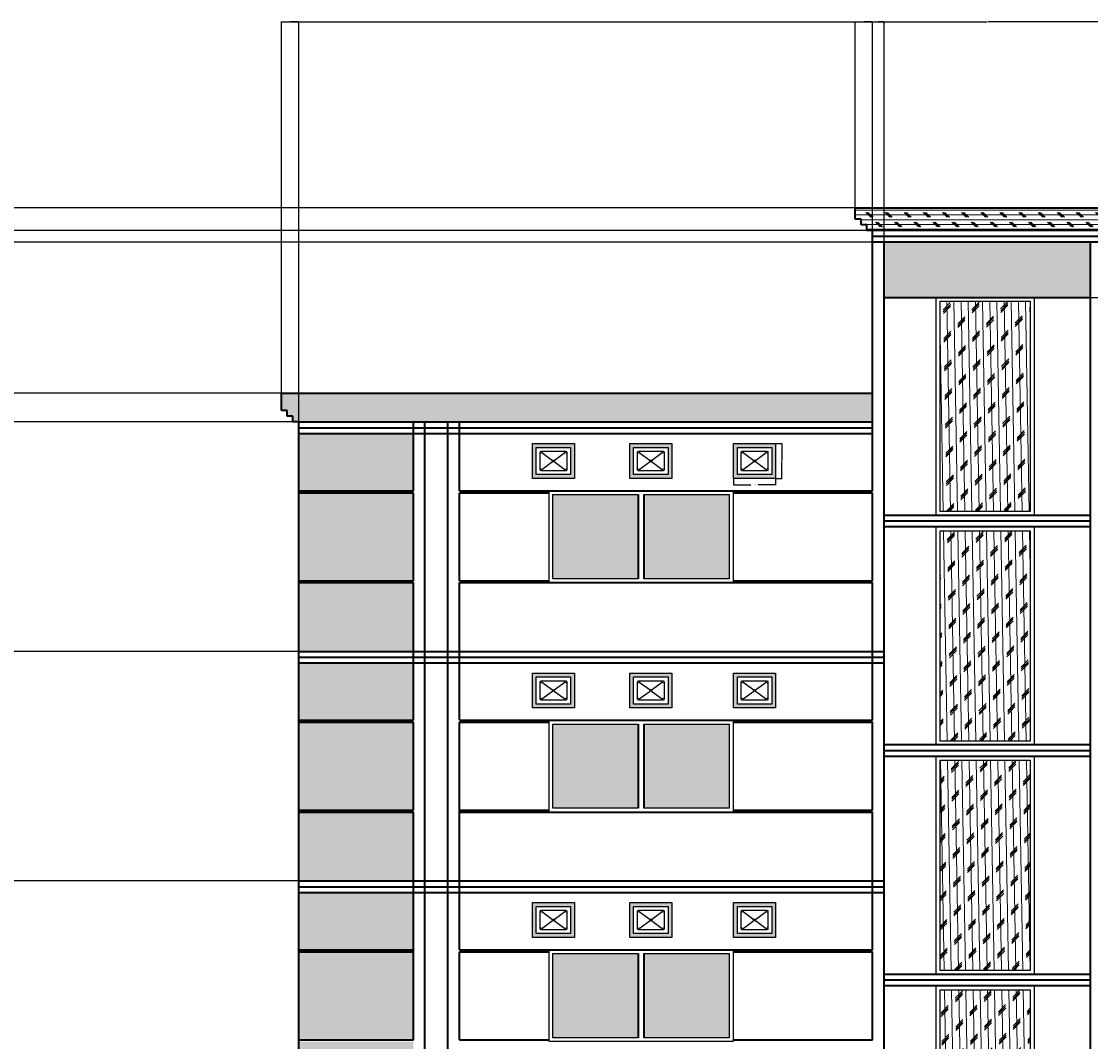
# Model space of a CAD drawing. Units: inches. Extents: x -742 to 1386, y -64 to 951.
# Tile 6 of 8: x -183 to 376, y 418 to 951. Entities that reach past the tile are written whole.
import ezdxf

# ---------------------------------------------------------------- set-up
doc = ezdxf.new("R2010")
doc.units = ezdxf.units.IN
doc.header["$MEASUREMENT"] = 0
for name, color, linetype, lineweight in [('A-ANNO-DIMS', 2, 'Continuous', 18), ('A-ELEV', 7, 'Continuous', 35), ('A-ELEV-PATT', 252, 'Continuous', 13), ('A-GLAZ', 4, 'Continuous', 25), ('A-GLAZ-PATT', 9, 'Continuous', 13), ('A-WALL-PATT', 8, 'Continuous', 13)]:
    doc.layers.add(name, color=color, linetype=linetype, lineweight=lineweight)
doc.styles.get("Standard").update_dxf_attribs({"font": 'arial.ttf'})
doc.dimstyles.get("Standard").update_dxf_attribs({"dimtxt": 0.18, "dimasz": 0.18, "dimexe": 0.18, "dimexo": 0.0625, "dimgap": 0.09, "dimtad": 0, "dimtih": 1, "dimtoh": 1, "dimdec": 4, "dimzin": 0, "dimdsep": 46, "dimtxsty": 'Standard', "dimcen": 0.09, "dimadec": 0, "dimazin": 0, "dimtfac": 1, "dimtdec": 4, "dimtofl": 0, "dimtmove": 0, "dimatfit": 3, "dimfxl": 1, "dimtolj": 1, "dimtzin": 0, "dimarcsym": 0})
pattern_1 = [(91, (0, 0), (-3.749429, -0.065447), []), (226, (1.842, 1.907), (7.62975, -7.36796), [5.3033, -5.3033]), (226, (1.826, 2.845), (7.62975, -7.36796), [5.3033, -5.3033]), (226, (1.809, 3.782), (7.62975, -7.36796), [5.3033, -5.3033])]

# ---------------------------------------------------------------- blocks, each defined once
blk = doc.blocks.new('VENT-WIN')
h = blk.add_hatch(color=256)
h.dxf.hatch_style = 1
h.paths.add_polyline_path([(11.51, 9.11, 1), (10.47, 9.11, 1)])
h.paths.add_polyline_path([(16.95, 13.71, 1), (17.99, 13.71, 1)])
h.paths.add_polyline_path([(17.99, 4.52, 1), (16.95, 4.52, 1)])
h.paths.add_polyline_path([(5.04, 4.52, 1), (4, 4.52, 1)])
h.paths.add_polyline_path([(4, 13.71, 1), (5.04, 13.71, 1)])
for p, q in [((4.99, 13.5), (10.57, 9.42)), ((11.41, 9.42), (16.99, 13.5)), ((4.99, 4.73), (10.57, 8.81)), ((11.41, 8.81), (16.99, 4.73))]:
    blk.add_line(p, q)
for points in [[(0, 18.22), (21.99, 18.22), (21.99, 0), (0, 0)], [(2, 16.22), (19.99, 16.22), (19.99, 2), (2, 2)]]:
    blk.add_lwpolyline(points, close=True)
for points in [[(4, 4.52), (4, 13.71)], [(4.52, 14.22), (17.47, 14.22)], [(17.99, 13.71), (17.99, 4.52)], [(17.47, 4), (4.52, 4)]]:
    blk.add_lwpolyline(points)
for centre in [(4.52, 13.71), (17.47, 13.71), (10.99, 9.11), (4.52, 4.52), (17.47, 4.52)]:
    blk.add_circle(centre, 0.519)
blk = doc.blocks.new('WIN-1000-2PANE')
blk.add_lwpolyline([(0, 48), (96.2, 48), (96.2, 0), (0, 0)], close=True)
for points in [[(46.6, 2), (2, 2), (2, 46), (46.6, 46)], [(49.6, 46), (94.2, 46), (94.2, 2), (49.6, 2)]]:
    blk.add_lwpolyline(points)
blk = doc.blocks.new('*D6')
at = {"layer": 'A-ANNO-DIMS', "color": 0, "lineweight": -2, "transparency": 16777216}
for p, q in [((189.57, 712.16), (189.57, 708.75)), ((211.56, 712.16), (211.56, 708.75)), ((189.75, 708.93), (198.62, 708.93)), ((211.38, 708.93), (202.51, 708.93))]:
    blk.add_line(p, q, dxfattribs=at)
at = {"layer": 'A-ANNO-DIMS', "color": 0, "transparency": 16777216}
for points in [[(189.75, 708.96), (189.75, 708.9), (189.57, 708.93)], [(211.38, 708.96), (211.38, 708.9), (211.56, 708.93)]]:
    blk.add_solid(points, dxfattribs=at)
at = {"layer": 'Defpoints', "color": 0, "transparency": 16777216}
for p in [(189.57, 712.23), (211.56, 712.23), (211.56, 708.93)]:
    blk.add_point(p, dxfattribs=at)
at = {"layer": 'A-ANNO-DIMS', "color": 0, "transparency": 16777216, "insert": (200.57, 708.93), "char_height": 0.18, "attachment_point": 5}
blk.add_mtext('\\A1;VENTILATOR WINDOW 22 TYP.', dxfattribs=at)
blk = doc.blocks.new('*D7')
at = {"layer": 'A-ANNO-DIMS', "color": 0, "lineweight": -2, "transparency": 16777216}
for p, q in [((211.62, 730.45), (215.04, 730.45)), ((214.86, 730.27), (214.86, 721.52)), ((214.86, 712.41), (214.86, 721.16)), ((211.62, 712.23), (215.04, 712.23))]:
    blk.add_line(p, q, dxfattribs=at)
at = {"layer": 'A-ANNO-DIMS', "color": 0, "transparency": 16777216}
for points in [[(214.83, 730.27), (214.89, 730.27), (214.86, 730.45)], [(214.83, 712.41), (214.89, 712.41), (214.86, 712.23)]]:
    blk.add_solid(points, dxfattribs=at)
at = {"layer": 'Defpoints', "color": 0, "transparency": 16777216}
for p in [(211.56, 730.45), (214.86, 730.45), (211.56, 712.23)]:
    blk.add_point(p, dxfattribs=at)
at = {"layer": 'A-ANNO-DIMS', "color": 0, "transparency": 16777216, "insert": (214.86, 721.34), "char_height": 0.18, "attachment_point": 5}
blk.add_mtext('\\A1;18 TYP.', dxfattribs=at)
blk = doc.blocks.new('*D10')
at = {"layer": 'A-ANNO-DIMS', "color": 0, "lineweight": -2, "transparency": 16777216}
for p, q in [((-46.77, 756.8), (-46.77, 951.21)), ((-46.59, 951.03), (321.94, 951.03)), ((691.05, 951.03), (322.52, 951.03)), ((691.23, 756.8), (691.23, 951.21))]:
    blk.add_line(p, q, dxfattribs=at)
at = {"layer": 'A-ANNO-DIMS', "color": 0, "transparency": 16777216}
for points in [[(-46.59, 951.06), (-46.59, 951), (-46.77, 951.03)], [(691.05, 951.06), (691.05, 951), (691.23, 951.03)]]:
    blk.add_solid(points, dxfattribs=at)
at = {"layer": 'Defpoints', "color": 0, "transparency": 16777216}
for p in [(691.23, 951.03), (-46.77, 756.74), (691.23, 756.74)]:
    blk.add_point(p, dxfattribs=at)
at = {"layer": 'A-ANNO-DIMS', "color": 0, "transparency": 16777216, "insert": (322.23, 951.03), "char_height": 0.18, "attachment_point": 5}
blk.add_mtext('\\A1;738', dxfattribs=at)
blk = doc.blocks.new('*D11')
at = {"layer": 'A-ANNO-DIMS', "color": 0, "lineweight": -2, "transparency": 16777216}
for p, q in [((253.23, 853.84), (253.23, 951.21)), ((253.41, 951.03), (321.95, 951.03)), ((391.05, 951.03), (322.51, 951.03)), ((391.23, 853.84), (391.23, 951.21))]:
    blk.add_line(p, q, dxfattribs=at)
at = {"layer": 'A-ANNO-DIMS', "color": 0, "transparency": 16777216}
for points in [[(253.41, 951.06), (253.41, 951), (253.23, 951.03)], [(391.05, 951.06), (391.05, 951), (391.23, 951.03)]]:
    blk.add_solid(points, dxfattribs=at)
at = {"layer": 'Defpoints', "color": 0, "transparency": 16777216}
for p in [(391.23, 951.03), (253.23, 853.78), (391.23, 853.78)]:
    blk.add_point(p, dxfattribs=at)
at = {"layer": 'A-ANNO-DIMS', "color": 0, "transparency": 16777216, "insert": (322.23, 951.03), "char_height": 0.18, "attachment_point": 5}
blk.add_mtext('\\A1;138', dxfattribs=at)
blk = doc.blocks.new('*D12')
at = {"layer": 'A-ANNO-DIMS', "color": 0, "lineweight": -2, "transparency": 16777216}
for p, q in [((-46.77, 747.8), (-46.77, 951.21)), ((-46.59, 951.03), (-42.42, 951.03)), ((-37.95, 951.03), (-42.12, 951.03)), ((-37.77, 741.8), (-37.77, 951.21))]:
    blk.add_line(p, q, dxfattribs=at)
at = {"layer": 'A-ANNO-DIMS', "color": 0, "transparency": 16777216}
for points in [[(-46.59, 951.06), (-46.59, 951), (-46.77, 951.03)], [(-37.95, 951.06), (-37.95, 951), (-37.77, 951.03)]]:
    blk.add_solid(points, dxfattribs=at)
at = {"layer": 'Defpoints', "color": 0, "transparency": 16777216}
for p in [(-37.77, 951.03), (-46.77, 747.74), (-37.77, 741.74)]:
    blk.add_point(p, dxfattribs=at)
at = {"layer": 'A-ANNO-DIMS', "color": 0, "transparency": 16777216, "insert": (-42.27, 951.03), "char_height": 0.18, "attachment_point": 5}
blk.add_mtext('\\A1;9', dxfattribs=at)
blk = doc.blocks.new('*D13')
at = {"layer": 'A-ANNO-DIMS', "color": 0, "lineweight": -2, "transparency": 16777216}
for p, q in [((253.23, 847.84), (253.23, 951.21)), ((253.41, 951.03), (257.58, 951.03)), ((262.05, 951.03), (257.88, 951.03)), ((262.23, 841.84), (262.23, 951.21))]:
    blk.add_line(p, q, dxfattribs=at)
at = {"layer": 'A-ANNO-DIMS', "color": 0, "transparency": 16777216}
for points in [[(253.41, 951.06), (253.41, 951), (253.23, 951.03)], [(262.05, 951.06), (262.05, 951), (262.23, 951.03)]]:
    blk.add_solid(points, dxfattribs=at)
at = {"layer": 'Defpoints', "color": 0, "transparency": 16777216}
for p in [(262.23, 951.03), (253.23, 847.78), (262.23, 841.78)]:
    blk.add_point(p, dxfattribs=at)
at = {"layer": 'A-ANNO-DIMS', "color": 0, "transparency": 16777216, "insert": (257.73, 951.03), "char_height": 0.18, "attachment_point": 5}
blk.add_mtext('\\A1;9', dxfattribs=at)
blk = doc.blocks.new('*D36')
at = {"layer": 'A-ANNO-DIMS', "color": 0, "lineweight": -2, "transparency": 16777216}
for p, q in [((262.23, 835.84), (262.23, 951.21)), ((262.41, 951.03), (265.08, 951.03)), ((268.05, 951.03), (265.38, 951.03)), ((268.23, 835.84), (268.23, 951.21))]:
    blk.add_line(p, q, dxfattribs=at)
at = {"layer": 'A-ANNO-DIMS', "color": 0, "transparency": 16777216}
for points in [[(262.41, 951.06), (262.41, 951), (262.23, 951.03)], [(268.05, 951.06), (268.05, 951), (268.23, 951.03)]]:
    blk.add_solid(points, dxfattribs=at)
at = {"layer": 'Defpoints', "color": 0, "transparency": 16777216}
for p in [(268.23, 951.03), (262.23, 835.78), (268.23, 835.78)]:
    blk.add_point(p, dxfattribs=at)
at = {"layer": 'A-ANNO-DIMS', "color": 0, "transparency": 16777216, "insert": (265.23, 951.03), "char_height": 0.18, "attachment_point": 5}
blk.add_mtext('\\A1;6', dxfattribs=at)
blk = doc.blocks.new('*D40')
at = {"layer": 'A-ANNO-DIMS', "color": 0, "lineweight": -2, "transparency": 16777216}
for p, q in [((-46.83, 756.74), (-741.55, 756.74)), ((-741.37, 756.56), (-741.37, 431.42)), ((-741.37, 105.92), (-741.37, 431.06)), ((-37.83, 105.74), (-741.55, 105.74))]:
    blk.add_line(p, q, dxfattribs=at)
at = {"layer": 'A-ANNO-DIMS', "color": 0, "transparency": 16777216}
for points in [[(-741.4, 756.56), (-741.34, 756.56), (-741.37, 756.74)], [(-741.4, 105.92), (-741.34, 105.92), (-741.37, 105.74)]]:
    blk.add_solid(points, dxfattribs=at)
at = {"layer": 'Defpoints', "color": 0, "transparency": 16777216}
for p in [(-46.77, 756.74), (-741.37, 105.74), (-37.77, 105.74)]:
    blk.add_point(p, dxfattribs=at)
at = {"layer": 'A-ANNO-DIMS', "color": 0, "transparency": 16777216, "insert": (-741.37, 431.24), "char_height": 0.18, "attachment_point": 5}
blk.add_mtext('\\A1;651', dxfattribs=at)
blk = doc.blocks.new('*D45')
at = {"layer": 'A-ANNO-DIMS', "color": 0, "lineweight": -2, "transparency": 16777216}
for p, q in [((-37.83, 501.74), (-741.55, 501.74)), ((-741.37, 501.56), (-741.37, 441.92)), ((-741.37, 381.92), (-741.37, 441.56)), ((-37.83, 381.74), (-741.55, 381.74))]:
    blk.add_line(p, q, dxfattribs=at)
at = {"layer": 'A-ANNO-DIMS', "color": 0, "transparency": 16777216}
for points in [[(-741.4, 501.56), (-741.34, 501.56), (-741.37, 501.74)], [(-741.4, 381.92), (-741.34, 381.92), (-741.37, 381.74)]]:
    blk.add_solid(points, dxfattribs=at)
at = {"layer": 'Defpoints', "color": 0, "transparency": 16777216}
for p in [(-741.37, 501.74), (-37.77, 501.74), (-37.77, 381.74)]:
    blk.add_point(p, dxfattribs=at)
at = {"layer": 'A-ANNO-DIMS', "color": 0, "transparency": 16777216, "insert": (-741.37, 441.74), "char_height": 0.18, "attachment_point": 5}
blk.add_mtext('\\A1;120', dxfattribs=at)
blk = doc.blocks.new('*D46')
at = {"layer": 'A-ANNO-DIMS', "color": 0, "lineweight": -2, "transparency": 16777216}
for p, q in [((-37.83, 621.74), (-741.55, 621.74)), ((-741.37, 621.56), (-741.37, 561.92)), ((-741.37, 501.92), (-741.37, 561.56)), ((-37.83, 501.74), (-741.55, 501.74))]:
    blk.add_line(p, q, dxfattribs=at)
at = {"layer": 'A-ANNO-DIMS', "color": 0, "transparency": 16777216}
for points in [[(-741.4, 621.56), (-741.34, 621.56), (-741.37, 621.74)], [(-741.4, 501.92), (-741.34, 501.92), (-741.37, 501.74)]]:
    blk.add_solid(points, dxfattribs=at)
at = {"layer": 'Defpoints', "color": 0, "transparency": 16777216}
for p in [(-741.37, 621.74), (-37.77, 621.74), (-37.77, 501.74)]:
    blk.add_point(p, dxfattribs=at)
at = {"layer": 'A-ANNO-DIMS', "color": 0, "transparency": 16777216, "insert": (-741.37, 561.74), "char_height": 0.18, "attachment_point": 5}
blk.add_mtext('\\A1;120', dxfattribs=at)
blk = doc.blocks.new('*D47')
at = {"layer": 'A-ANNO-DIMS', "color": 0, "lineweight": -2, "transparency": 16777216}
for p, q in [((-37.83, 741.74), (-741.55, 741.74)), ((-741.37, 741.56), (-741.37, 681.92)), ((-741.37, 621.92), (-741.37, 681.56)), ((-37.83, 621.74), (-741.55, 621.74))]:
    blk.add_line(p, q, dxfattribs=at)
at = {"layer": 'A-ANNO-DIMS', "color": 0, "transparency": 16777216}
for points in [[(-741.4, 741.56), (-741.34, 741.56), (-741.37, 741.74)], [(-741.4, 621.92), (-741.34, 621.92), (-741.37, 621.74)]]:
    blk.add_solid(points, dxfattribs=at)
at = {"layer": 'Defpoints', "color": 0, "transparency": 16777216}
for p in [(-741.37, 741.74), (-37.77, 741.74), (-37.77, 621.74)]:
    blk.add_point(p, dxfattribs=at)
at = {"layer": 'A-ANNO-DIMS', "color": 0, "transparency": 16777216, "insert": (-741.37, 681.74), "char_height": 0.18, "attachment_point": 5}
blk.add_mtext('\\A1;120', dxfattribs=at)
blk = doc.blocks.new('*D48')
at = {"layer": 'A-ANNO-DIMS', "color": 0, "lineweight": -2, "transparency": 16777216}
for p, q in [((-46.83, 756.74), (-741.55, 756.74)), ((-741.37, 756.56), (-741.37, 749.42)), ((-741.37, 741.92), (-741.37, 749.06)), ((-37.83, 741.74), (-741.55, 741.74))]:
    blk.add_line(p, q, dxfattribs=at)
at = {"layer": 'A-ANNO-DIMS', "color": 0, "transparency": 16777216}
for points in [[(-741.4, 756.56), (-741.34, 756.56), (-741.37, 756.74)], [(-741.4, 741.92), (-741.34, 741.92), (-741.37, 741.74)]]:
    blk.add_solid(points, dxfattribs=at)
at = {"layer": 'Defpoints', "color": 0, "transparency": 16777216}
for p in [(-741.37, 756.74), (-46.77, 756.74), (-37.77, 741.74)]:
    blk.add_point(p, dxfattribs=at)
at = {"layer": 'A-ANNO-DIMS', "color": 0, "transparency": 16777216, "insert": (-741.37, 749.24), "char_height": 0.18, "attachment_point": 5}
blk.add_mtext('\\A1;15', dxfattribs=at)
blk = doc.blocks.new('*D52')
at = {"layer": 'A-ANNO-DIMS', "color": 0, "lineweight": -2, "transparency": 16777216}
for p, q in [((253.17, 853.78), (-741.55, 853.78)), ((-741.37, 853.6), (-741.37, 805.44)), ((-741.37, 756.92), (-741.37, 805.08)), ((262.17, 756.74), (-741.55, 756.74))]:
    blk.add_line(p, q, dxfattribs=at)
at = {"layer": 'A-ANNO-DIMS', "color": 0, "transparency": 16777216}
for points in [[(-741.4, 853.6), (-741.34, 853.6), (-741.37, 853.78)], [(-741.4, 756.92), (-741.34, 756.92), (-741.37, 756.74)]]:
    blk.add_solid(points, dxfattribs=at)
at = {"layer": 'Defpoints', "color": 0, "transparency": 16777216}
for p in [(-741.37, 853.78), (253.23, 853.78), (262.23, 756.74)]:
    blk.add_point(p, dxfattribs=at)
at = {"layer": 'A-ANNO-DIMS', "color": 0, "transparency": 16777216, "insert": (-741.37, 805.26), "char_height": 0.18, "attachment_point": 5}
blk.add_mtext('\\A1;97.04', dxfattribs=at)
blk = doc.blocks.new('*D53')
at = {"layer": 'A-ANNO-DIMS', "color": 0, "lineweight": -2, "transparency": 16777216}
for p, q in [((253.17, 853.78), (-741.55, 853.78)), ((-741.37, 853.6), (-741.37, 847.96)), ((-741.37, 841.96), (-741.37, 847.6)), ((262.17, 841.78), (-741.55, 841.78))]:
    blk.add_line(p, q, dxfattribs=at)
at = {"layer": 'A-ANNO-DIMS', "color": 0, "transparency": 16777216}
for points in [[(-741.4, 853.6), (-741.34, 853.6), (-741.37, 853.78)], [(-741.4, 841.96), (-741.34, 841.96), (-741.37, 841.78)]]:
    blk.add_solid(points, dxfattribs=at)
at = {"layer": 'Defpoints', "color": 0, "transparency": 16777216}
for p in [(253.23, 853.78), (-741.37, 841.78), (262.23, 841.78)]:
    blk.add_point(p, dxfattribs=at)
at = {"layer": 'A-ANNO-DIMS', "color": 0, "transparency": 16777216, "insert": (-741.37, 847.78), "char_height": 0.18, "attachment_point": 5}
blk.add_mtext('\\A1;12', dxfattribs=at)
blk = doc.blocks.new('*D54')
at = {"layer": 'A-ANNO-DIMS', "color": 0, "lineweight": -2, "transparency": 16777216}
for p, q in [((262.17, 841.78), (-741.55, 841.78)), ((-741.37, 841.6), (-741.37, 838.96)), ((-741.37, 835.96), (-741.37, 838.6)), ((262.17, 835.78), (-741.55, 835.78))]:
    blk.add_line(p, q, dxfattribs=at)
at = {"layer": 'A-ANNO-DIMS', "color": 0, "transparency": 16777216}
for points in [[(-741.4, 841.6), (-741.34, 841.6), (-741.37, 841.78)], [(-741.4, 835.96), (-741.34, 835.96), (-741.37, 835.78)]]:
    blk.add_solid(points, dxfattribs=at)
at = {"layer": 'Defpoints', "color": 0, "transparency": 16777216}
for p in [(262.23, 841.78), (-741.37, 835.78), (262.23, 835.78)]:
    blk.add_point(p, dxfattribs=at)
at = {"layer": 'A-ANNO-DIMS', "color": 0, "transparency": 16777216, "insert": (-741.37, 838.78), "char_height": 0.18, "attachment_point": 5}
blk.add_mtext('\\A1;6', dxfattribs=at)
blk = doc.blocks.new('*D57')
at = {"layer": 'A-ANNO-DIMS', "color": 0, "lineweight": -2, "transparency": 16777216}
for p, q in [((376.29, 835.78), (1386.01, 835.78)), ((1385.83, 835.6), (1385.83, 821.5)), ((1385.83, 807.03), (1385.83, 821.14)), ((346.76, 806.85), (1386.01, 806.85))]:
    blk.add_line(p, q, dxfattribs=at)
at = {"layer": 'A-ANNO-DIMS', "color": 0, "transparency": 16777216}
for points in [[(1385.8, 835.6), (1385.86, 835.6), (1385.83, 835.78)], [(1385.8, 807.03), (1385.86, 807.03), (1385.83, 806.85)]]:
    blk.add_solid(points, dxfattribs=at)
at = {"layer": 'Defpoints', "color": 0, "transparency": 16777216}
for p in [(376.23, 835.78), (1385.83, 835.78), (346.7, 806.85)]:
    blk.add_point(p, dxfattribs=at)
at = {"layer": 'A-ANNO-DIMS', "color": 0, "transparency": 16777216, "insert": (1385.83, 821.32), "char_height": 0.18, "attachment_point": 5}
blk.add_mtext('\\A1;28.925', dxfattribs=at)

msp = doc.modelspace()

# ---------------------------------------------------------------- hatches: boundary and pattern name
at = {"layer": 'A-ELEV-PATT'}
h = msp.add_hatch(color=256, dxfattribs=at)
h.dxf.hatch_style = 1
h.paths.add_polyline_path([(106.4136, 730.4496), (84.4263, 730.4496), (84.4263, 712.2254), (106.4136, 712.2254)])
h.paths.add_polyline_path([(104.4136, 714.2254), (86.4263, 714.2254), (86.4263, 728.4496), (104.4136, 728.4496)], flags=16)
h.paths.add_polyline_path([(157.3109, 730.4496), (135.3236, 730.4496), (135.3236, 712.2254), (157.3109, 712.2254)])
h.paths.add_polyline_path([(155.3109, 728.4496), (155.3109, 714.2254), (137.3236, 714.2254), (137.3236, 728.4496)], flags=16)
h.paths.add_polyline_path([(211.5617, 730.4496), (189.5743, 730.4496), (189.5743, 712.2254), (211.5617, 712.2254)])
h.paths.add_polyline_path([(209.5617, 728.4496), (209.5617, 714.2254), (191.5743, 714.2254), (191.5743, 728.4496)], flags=16)
h = msp.add_hatch(color=256, dxfattribs=at)
h.dxf.hatch_style = 1
h.set_gradient(color1=(0, 255, 255), name='CURVED')
h.paths.add_polyline_path([(139.7128, 703.7399), (95.1117, 703.7399), (95.1117, 659.7399), (139.7128, 659.7399)])
h.paths.add_polyline_path([(187.3139, 703.7399), (142.7128, 703.7399), (142.7128, 659.7399), (187.3139, 659.7399)])
h.paths.add_polyline_path([(501.7423, 703.7399), (457.1413, 703.7399), (457.1413, 659.7399), (501.7423, 659.7399)])
h.paths.add_polyline_path([(549.3434, 703.7399), (504.7423, 703.7399), (504.7423, 659.7399), (549.3434, 659.7399)])
h = msp.add_hatch(color=256, dxfattribs=at)
h.dxf.hatch_style = 1
h.paths.add_polyline_path([(106.4136, 610.4496), (84.4263, 610.4496), (84.4263, 592.2254), (106.4136, 592.2254)])
h.paths.add_polyline_path([(104.4136, 594.2254), (86.4263, 594.2254), (86.4263, 608.4496), (104.4136, 608.4496)], flags=16)
h.paths.add_polyline_path([(157.3109, 610.4496), (135.3236, 610.4496), (135.3236, 592.2254), (157.3109, 592.2254)])
h.paths.add_polyline_path([(155.3109, 608.4496), (155.3109, 594.2254), (137.3236, 594.2254), (137.3236, 608.4496)], flags=16)
h.paths.add_polyline_path([(211.5617, 610.4496), (189.5743, 610.4496), (189.5743, 592.2254), (211.5617, 592.2254)])
h.paths.add_polyline_path([(209.5617, 608.4496), (209.5617, 594.2254), (191.5743, 594.2254), (191.5743, 608.4496)], flags=16)
h = msp.add_hatch(color=256, dxfattribs=at)
h.dxf.hatch_style = 1
h.set_gradient(color1=(0, 255, 255), name='CURVED')
h.paths.add_polyline_path([(139.7128, 583.7399), (95.1117, 583.7399), (95.1117, 539.7399), (139.7128, 539.7399)])
h.paths.add_polyline_path([(187.3139, 583.7399), (142.7128, 583.7399), (142.7128, 539.7399), (187.3139, 539.7399)])
h.paths.add_polyline_path([(501.7423, 583.7399), (457.1413, 583.7399), (457.1413, 539.7399), (501.7423, 539.7399)])
h.paths.add_polyline_path([(549.3434, 583.7399), (504.7423, 583.7399), (504.7423, 539.7399), (549.3434, 539.7399)])
h = msp.add_hatch(color=256, dxfattribs=at)
h.dxf.hatch_style = 1
h.paths.add_polyline_path([(106.4136, 490.4496), (84.4263, 490.4496), (84.4263, 472.2254), (106.4136, 472.2254)])
h.paths.add_polyline_path([(104.4136, 474.2254), (86.4263, 474.2254), (86.4263, 488.4496), (104.4136, 488.4496)], flags=16)
h.paths.add_polyline_path([(157.3109, 490.4496), (135.3236, 490.4496), (135.3236, 472.2254), (157.3109, 472.2254)])
h.paths.add_polyline_path([(155.3109, 488.4496), (155.3109, 474.2254), (137.3236, 474.2254), (137.3236, 488.4496)], flags=16)
h.paths.add_polyline_path([(211.5617, 490.4496), (189.5743, 490.4496), (189.5743, 472.2254), (211.5617, 472.2254)])
h.paths.add_polyline_path([(209.5617, 488.4496), (209.5617, 474.2254), (191.5743, 474.2254), (191.5743, 488.4496)], flags=16)
h = msp.add_hatch(color=256, dxfattribs=at)
h.dxf.hatch_style = 1
h.set_gradient(color1=(0, 255, 255), name='CURVED')
h.paths.add_polyline_path([(139.7128, 463.7399), (95.1117, 463.7399), (95.1117, 419.7399), (139.7128, 419.7399)])
h.paths.add_polyline_path([(187.3139, 463.7399), (142.7128, 463.7399), (142.7128, 419.7399), (187.3139, 419.7399)])
h.paths.add_polyline_path([(501.7423, 463.7399), (457.1413, 463.7399), (457.1413, 419.7399), (501.7423, 419.7399)])
h.paths.add_polyline_path([(549.3434, 463.7399), (504.7423, 463.7399), (504.7423, 419.7399), (549.3434, 419.7399)])
at = {"layer": 'A-GLAZ-PATT', "transparency": 33554457}
h = msp.add_hatch(dxfattribs=at)
h.set_pattern_fill('CORK', color=256, scale=30, angle=91)
h.set_pattern_definition(pattern_1)
h.paths.add_polyline_path([(344.6973, 804.8548), (297.5643, 804.8548), (297.5643, 694.8548), (344.6973, 694.8548)])
h = msp.add_hatch(dxfattribs=at)
h.set_pattern_fill('CORK', color=256, scale=30, angle=91)
h.set_pattern_definition(pattern_1)
h.paths.add_polyline_path([(344.6973, 684.8548), (297.5643, 684.8548), (297.5643, 574.8548), (344.6973, 574.8548)])
h = msp.add_hatch(dxfattribs=at)
h.set_pattern_fill('CORK', color=256, scale=30, angle=91)
h.set_pattern_definition(pattern_1)
h.paths.add_polyline_path([(344.6973, 564.8548), (297.5643, 564.8548), (297.5643, 454.8548), (344.6973, 454.8548)])
h = msp.add_hatch(dxfattribs=at)
h.set_pattern_fill('CORK', color=256, scale=30, angle=91)
h.set_pattern_definition(pattern_1)
h.paths.add_polyline_path([(344.6973, 444.8548), (297.5643, 444.8548), (297.5643, 334.8548), (344.6973, 334.8548)])
at = {"layer": 'A-WALL-PATT', "transparency": 33554457}
h = msp.add_hatch(dxfattribs=at)
h.set_pattern_fill('CORK', color=256, scale=20)
h.set_pattern_definition([(0, (0, 0), (0, 2.5), []), (135, (1.25, -1.25), (-5, -5), [3.535534, -3.535534]), (135, (1.875, -1.25), (-5, -5), [3.535534, -3.535534]), (135, (2.5, -1.25), (-5, -5), [3.535534, -3.535534])])
h.paths.add_polyline_path([(382.2276, 841.7799), (385.2276, 841.7799), (385.2276, 844.7799), (388.2276, 844.7799), (388.2276, 847.7799), (391.2276, 847.7799), (391.2276, 853.7799), (253.2276, 853.7799), (253.2276, 847.7799), (256.2276, 847.7799), (256.2276, 844.7799), (259.2276, 844.7799), (259.2276, 841.7799), (262.2276, 841.7799)])
h = msp.add_hatch(dxfattribs=at)
h.set_pattern_fill('AR-B88', color=256)
h.paths.add_polyline_path([(22.2276, 224.7399), (-37.7724, 224.7399), (-37.7724, 178.7399), (22.2276, 178.7399)])
h.paths.add_polyline_path([(22.2276, 177.7399), (-37.7724, 177.7399), (-37.7724, 141.7399), (22.2276, 141.7399)])
h.paths.add_polyline_path([(22.2276, 255.7399), (-37.7724, 255.7399), (-37.7724, 225.7399), (22.2276, 225.7399)])
h.paths.add_polyline_path([(22.2276, 297.7399), (-37.7724, 297.7399), (-37.7724, 261.7399), (22.2276, 261.7399)])
h.paths.add_polyline_path([(22.2276, 344.7399), (-37.7724, 344.7399), (-37.7724, 298.7399), (22.2276, 298.7399)])
h.paths.add_polyline_path([(22.2276, 375.7399), (-37.7724, 375.7399), (-37.7724, 345.7399), (22.2276, 345.7399)])
h.paths.add_polyline_path([(22.2276, 417.7399), (-37.7724, 417.7399), (-37.7724, 381.7399), (22.2276, 381.7399)])
h.paths.add_polyline_path([(22.2276, 464.7399), (-37.7724, 464.7399), (-37.7724, 418.7399), (22.2276, 418.7399)])
h.paths.add_polyline_path([(22.2276, 495.7399), (-37.7724, 495.7399), (-37.7724, 465.7399), (22.2276, 465.7399)])
h.paths.add_polyline_path([(22.2276, 537.7399), (-37.7724, 537.7399), (-37.7724, 501.7399), (22.2276, 501.7399)])
h.paths.add_polyline_path([(22.2276, 584.7399), (-37.7724, 584.7399), (-37.7724, 538.7399), (22.2276, 538.7399)])
h.paths.add_polyline_path([(22.2276, 615.7399), (-37.7724, 615.7399), (-37.7724, 585.7399), (22.2276, 585.7399)])
h.paths.add_polyline_path([(22.2276, 657.7399), (-37.7724, 657.7399), (-37.7724, 621.7399), (22.2276, 621.7399)])
h.paths.add_polyline_path([(22.2276, 704.7399), (-37.7724, 704.7399), (-37.7724, 658.7399), (22.2276, 658.7399)])
h.paths.add_polyline_path([(22.2276, 735.7399), (-37.7724, 735.7399), (-37.7724, 705.7399), (22.2276, 705.7399)])
h.paths.add_polyline_path([(376.2276, 835.7799), (268.2276, 835.7799), (268.2276, 806.8548), (376.2276, 806.8548)])
h.paths.add_polyline_path([(682.2276, 735.7399), (622.2276, 735.7399), (622.2276, 705.7399), (682.2276, 705.7399)])
h.paths.add_polyline_path([(682.2276, 704.7399), (622.2276, 704.7399), (622.2276, 658.7399), (682.2276, 658.7399)])
h.paths.add_polyline_path([(682.2276, 657.7399), (622.2276, 657.7399), (622.2276, 621.7399), (682.2276, 621.7399)])
h.paths.add_polyline_path([(682.2276, 615.7399), (622.2276, 615.7399), (622.2276, 585.7399), (682.2276, 585.7399)])
h.paths.add_polyline_path([(682.2276, 584.7399), (622.2276, 584.7399), (622.2276, 538.7399), (682.2276, 538.7399)])
h.paths.add_polyline_path([(682.2276, 537.7399), (622.2276, 537.7399), (622.2276, 501.7399), (682.2276, 501.7399)])
h.paths.add_polyline_path([(682.2276, 495.7399), (622.2276, 495.7399), (622.2276, 465.7399), (682.2276, 465.7399)])
h.paths.add_polyline_path([(682.2276, 464.7399), (622.2276, 464.7399), (622.2276, 418.7399), (682.2276, 418.7399)])
h.paths.add_polyline_path([(682.2276, 417.7399), (622.2276, 417.7399), (622.2276, 381.7399), (682.2276, 381.7399)])
h.paths.add_polyline_path([(682.2276, 375.7399), (622.2276, 375.7399), (622.2276, 345.7399), (682.2276, 345.7399)])
h.paths.add_polyline_path([(682.2276, 344.7399), (622.2276, 344.7399), (622.2276, 298.7399), (682.2276, 298.7399)])
h.paths.add_polyline_path([(682.2276, 297.7399), (622.2276, 297.7399), (622.2276, 261.7399), (682.2276, 261.7399)])
h.paths.add_polyline_path([(682.2276, 255.7399), (622.2276, 255.7399), (622.2276, 225.7399), (682.2276, 225.7399)])
h.paths.add_polyline_path([(682.2276, 224.7399), (622.2276, 224.7399), (622.2276, 178.7399), (682.2276, 178.7399)])
h.paths.add_polyline_path([(682.2276, 177.7399), (622.2276, 177.7399), (622.2276, 141.7399), (682.2276, 141.7399)])
h = msp.add_hatch(dxfattribs=at)
h.set_pattern_fill('CORK', color=256, scale=30, angle=91)
h.set_pattern_definition(pattern_1)
h.paths.add_polyline_path([(262.2276, 756.7399), (-46.7724, 756.7399), (-46.7724, 753.7399), (-46.7724, 747.7399), (-43.7724, 747.7399), (-43.7724, 744.7399), (-40.7724, 744.7399), (-40.7724, 741.7399), (-37.7724, 741.7399), (262.2276, 741.7399)])
h.paths.add_polyline_path([(688.2276, 747.7399), (691.2276, 747.7399), (691.2276, 753.7399), (691.2276, 756.7399), (382.2276, 756.7399), (382.2276, 741.7399), (682.2276, 741.7399), (685.2276, 741.7399), (685.2276, 744.7399), (688.2276, 744.7399)])

# ---------------------------------------------------------------- linework, layer by layer
at = {"layer": 'A-ELEV'}
for p, q in [((253.2276, 847.7799), (253.2276, 853.7799)), ((253.2276, 853.7799), (391.2276, 853.7799)), ((256.2276, 847.7799), (253.2276, 847.7799)), ((256.2276, 844.7799), (256.2276, 847.7799)), ((259.2276, 844.7799), (256.2276, 844.7799)), ((259.2276, 841.7799), (259.2276, 844.7799)), ((262.2276, 841.7799), (259.2276, 841.7799)), ((382.2276, 841.7799), (262.2276, 841.7799)), ((262.2276, 835.7799), (262.2276, 841.7799)), ((382.2276, 838.7799), (262.2276, 838.7799)), ((262.2276, 705.7399), (262.2276, 835.7799)), ((382.2276, 835.7799), (262.2276, 835.7799)), ((268.2276, 105.7399), (268.2276, 835.7799)), ((376.2276, 105.7399), (376.2276, 835.7799)), ((268.2276, 806.8548), (376.2276, 806.8548)), ((-46.7724, 753.7399), (-46.7724, 756.7399)), ((-46.7724, 756.7399), (262.2276, 756.7399)), ((-46.7724, 747.7399), (-46.7724, 753.7399)), ((-43.7724, 747.7399), (-46.7724, 747.7399)), ((-43.7724, 744.7399), (-43.7724, 747.7399)), ((-40.7724, 744.7399), (-43.7724, 744.7399)), ((-40.7724, 741.7399), (-40.7724, 744.7399)), ((-37.7724, 741.7399), (-40.7724, 741.7399)), ((-37.7724, 741.7399), (262.2276, 741.7399)), ((-37.7724, 141.7399), (-37.7724, 741.7399)), ((-37.7724, 738.7399), (262.2276, 738.7399)), ((22.2276, 705.7399), (22.2276, 741.7399)), ((28.2276, 141.7399), (28.2276, 741.7399)), ((40.2276, 141.7399), (40.2276, 741.7399)), ((46.2276, 705.7399), (46.2276, 741.7399)), ((-37.7724, 735.7399), (262.2276, 735.7399)), ((-37.7724, 705.7399), (22.2276, 705.7399)), ((-37.7724, 704.7399), (22.2276, 704.7399)), ((22.2276, 658.7399), (22.2276, 704.7399)), ((46.2276, 705.7399), (262.2276, 705.7399)), ((46.2276, 704.7399), (93.1117, 704.7399)), ((46.2276, 658.7399), (46.2276, 704.7399)), ((189.3139, 704.7399), (262.2276, 704.7399)), ((262.2276, 658.7399), (262.2276, 704.7399)), ((139.7128, 703.7399), (139.7128, 659.7399)), ((142.7128, 703.7399), (142.7128, 659.7399)), ((376.2276, 692.8548), (268.2276, 692.8548)), ((376.2276, 689.8548), (268.2276, 689.8548)), ((376.2276, 686.8548), (268.2276, 686.8548)), ((-37.7724, 658.7399), (22.2276, 658.7399)), ((-37.7724, 657.7399), (22.2276, 657.7399)), ((22.2276, 585.7399), (22.2276, 657.7399)), ((46.2276, 658.7399), (93.1117, 658.7399)), ((46.2276, 657.7399), (262.2276, 657.7399)), ((46.2276, 585.7399), (46.2276, 657.7399)), ((189.3139, 658.7399), (262.2276, 658.7399)), ((262.2276, 585.7399), (262.2276, 657.7399)), ((-37.7724, 621.7399), (268.2276, 621.7399)), ((-37.7724, 618.7399), (268.2276, 618.7399)), ((-37.7724, 615.7399), (268.2276, 615.7399)), ((-37.7724, 585.7399), (22.2276, 585.7399)), ((-37.7724, 584.7399), (22.2276, 584.7399)), ((22.2276, 538.7399), (22.2276, 584.7399)), ((46.2276, 585.7399), (262.2276, 585.7399)), ((46.2276, 584.7399), (93.1117, 584.7399)), ((46.2276, 465.7399), (46.2276, 584.7399)), ((139.7128, 583.7399), (139.7128, 539.7399)), ((142.7128, 583.7399), (142.7128, 539.7399)), ((189.3139, 584.7399), (262.2276, 584.7399)), ((262.2276, 538.7399), (262.2276, 584.7399)), ((376.2276, 572.8548), (268.2276, 572.8548)), ((376.2276, 569.8548), (268.2276, 569.8548)), ((376.2276, 566.8548), (268.2276, 566.8548)), ((-37.7724, 538.7399), (22.2276, 538.7399)), ((-37.7724, 537.7399), (22.2276, 537.7399)), ((22.2276, 418.7399), (22.2276, 537.7399)), ((46.2276, 538.7399), (93.1117, 538.7399)), ((46.2276, 537.7399), (262.2276, 537.7399)), ((189.3139, 538.7399), (262.2276, 538.7399)), ((262.2276, 465.7399), (262.2276, 537.7399)), ((-37.7724, 501.7399), (268.2276, 501.7399)), ((-37.7724, 498.7399), (268.2276, 498.7399)), ((-37.7724, 495.7399), (268.2276, 495.7399)), ((-37.7724, 465.7399), (22.2276, 465.7399)), ((-37.7724, 464.7399), (22.2276, 464.7399)), ((46.2276, 465.7399), (262.2276, 465.7399)), ((46.2276, 464.7399), (93.1117, 464.7399)), ((46.2276, 418.7399), (46.2276, 464.7399)), ((189.3139, 464.7399), (262.2276, 464.7399)), ((262.2276, 418.7399), (262.2276, 464.7399)), ((139.7128, 463.7399), (139.7128, 419.7399)), ((142.7128, 463.7399), (142.7128, 419.7399)), ((376.2276, 452.8548), (268.2276, 452.8548)), ((376.2276, 449.8548), (268.2276, 449.8548)), ((376.2276, 446.8548), (268.2276, 446.8548)), ((-37.7724, 418.7399), (22.2276, 418.7399)), ((46.2276, 418.7399), (93.1117, 418.7399)), ((189.3139, 418.7399), (262.2276, 418.7399))]:
    msp.add_line(p, q, dxfattribs=at)
at = {"layer": 'A-GLAZ'}
for points in [[(295.5643, 806.8548), (346.6973, 806.8548), (346.6973, 692.8548), (295.5643, 692.8548)], [(297.5643, 804.8548), (344.6973, 804.8548), (344.6973, 694.8548), (297.5643, 694.8548)], [(295.5643, 686.8548), (346.6973, 686.8548), (346.6973, 572.8548), (295.5643, 572.8548)], [(297.5643, 684.8548), (344.6973, 684.8548), (344.6973, 574.8548), (297.5643, 574.8548)], [(295.5643, 566.8548), (346.6973, 566.8548), (346.6973, 452.8548), (295.5643, 452.8548)], [(297.5643, 564.8548), (344.6973, 564.8548), (344.6973, 454.8548), (297.5643, 454.8548)], [(295.5643, 446.8548), (346.6973, 446.8548), (346.6973, 332.8548), (295.5643, 332.8548)], [(297.5643, 444.8548), (344.6973, 444.8548), (344.6973, 334.8548), (297.5643, 334.8548)]]:
    msp.add_lwpolyline(points, close=True, dxfattribs=at)

# ---------------------------------------------------------------- block references
for name, p in [('VENT-WIN', (84.4267, 712.225)), ('VENT-WIN', (135.324, 712.225)), ('VENT-WIN', (189.5748, 712.225)), ('WIN-1000-2PANE', (93.112, 657.74)), ('VENT-WIN', (84.4267, 592.225)), ('VENT-WIN', (135.324, 592.225)), ('VENT-WIN', (189.5748, 592.225)), ('WIN-1000-2PANE', (93.112, 537.74)), ('VENT-WIN', (84.4267, 472.225)), ('VENT-WIN', (135.324, 472.225)), ('VENT-WIN', (189.5748, 472.225)), ('WIN-1000-2PANE', (93.112, 417.74))]:
    msp.add_blockref(name, p, dxfattribs=at)

# ---------------------------------------------------------------- dimensions: what is measured, and where the dimension line sits
at = {"layer": 'A-ANNO-DIMS'}
for base, p1, p2, picture, middle in [((691.2276, 951.0299), (-46.7724, 756.7399), (691.2276, 756.7399), '*D10', (322.2276, 951.0299)), ((-37.7724, 951.0299), (-46.7724, 747.7399), (-37.7724, 741.7399), '*D12', (-42.2724, 951.0299)), ((391.2276, 951.0299), (253.2276, 853.7799), (391.2276, 853.7799), '*D11', (322.2276, 951.0299)), ((262.2276, 951.0299), (253.2276, 847.7799), (262.2276, 841.7799), '*D13', (257.7276, 951.0299)), ((268.2276, 951.0299), (262.2276, 835.7799), (268.2276, 835.7799), '*D36', (265.2276, 951.0299))]:
    dim = msp.add_linear_dim(base=base, p1=p1, p2=p2, dimstyle='Standard', override={"dimdec": 0, "dimlfac": 1, "dimrnd": 0, "dimzin": 0, "dimdsep": 46, "dimlunit": 2}, dxfattribs=at)
    dim.commit()
    dim.dimension.update_dxf_attribs({"geometry": picture, "text_midpoint": middle})
for base, p1, p2, override, picture, middle in [((-741.3711, 853.7799), (262.2276, 756.7399), (253.2276, 853.7799), {"dimdec": 2, "dimlfac": 1, "dimrnd": 0, "dimzin": 0, "dimdsep": 46, "dimlunit": 2}, '*D52', (-741.3711, 805.2599)), ((-741.3711, 841.7799), (253.2276, 853.7799), (262.2276, 841.7799), {"dimdec": 0, "dimlfac": 1, "dimrnd": 0, "dimzin": 0, "dimdsep": 46, "dimlunit": 2}, '*D53', (-741.3711, 847.7799)), ((-741.3711, 835.7799), (262.2276, 841.7799), (262.2276, 835.7799), {"dimdec": 0, "dimlfac": 1, "dimrnd": 0, "dimzin": 0, "dimdsep": 46, "dimlunit": 2}, '*D54', (-741.3711, 838.7799)), ((1385.8262, 835.7799), (346.6973, 806.8548), (376.2276, 835.7799), {"dimdec": 3, "dimlfac": 1, "dimrnd": 0, "dimzin": 0, "dimdsep": 46, "dimlunit": 2}, '*D57', (1385.8262, 821.3173)), ((-741.3711, 105.7399), (-46.7724, 756.7399), (-37.7724, 105.7399), {"dimdec": 0, "dimlfac": 1, "dimrnd": 0, "dimzin": 0, "dimdsep": 46, "dimlunit": 2}, '*D40', (-741.3711, 431.2399)), ((-741.3711, 756.7399), (-37.7724, 741.7399), (-46.7724, 756.7399), {"dimdec": 0, "dimlfac": 1, "dimrnd": 0, "dimzin": 0, "dimdsep": 46, "dimlunit": 2}, '*D48', (-741.3711, 749.2399)), ((-741.3711, 741.7399), (-37.7724, 621.7399), (-37.7724, 741.7399), {"dimdec": 0, "dimlfac": 1, "dimrnd": 0, "dimzin": 0, "dimdsep": 46, "dimlunit": 2}, '*D47', (-741.3711, 681.7399)), ((-741.3711, 621.7399), (-37.7724, 501.7399), (-37.7724, 621.7399), {"dimdec": 0, "dimlfac": 1, "dimrnd": 0, "dimzin": 0, "dimdsep": 46, "dimlunit": 2}, '*D46', (-741.3711, 561.7399)), ((-741.3711, 501.7399), (-37.7724, 381.7399), (-37.7724, 501.7399), {"dimdec": 0, "dimlfac": 1, "dimrnd": 0, "dimzin": 0, "dimdsep": 46, "dimlunit": 2}, '*D45', (-741.3711, 441.7399))]:
    dim = msp.add_linear_dim(base=base, p1=p1, p2=p2, angle=90, dimstyle='Standard', override=override, dxfattribs=at)
    dim.commit()
    dim.dimension.update_dxf_attribs({"geometry": picture, "text_midpoint": middle})
dim = msp.add_linear_dim(base=(214.8598, 730.4496), p1=(211.5617, 712.2254), p2=(211.5617, 730.4496), angle=90, text='<> TYP.', dimstyle='Standard', override={"dimdec": 0, "dimrnd": 0, "dimzin": 0, "dimlunit": 2}, dxfattribs=at)
dim.commit()
dim.dimension.update_dxf_attribs({"geometry": '*D7', "text_midpoint": (214.8598, 721.3375)})
dim = msp.add_linear_dim(base=(211.5617, 708.9273), p1=(189.5743, 712.2254), p2=(211.5617, 712.2254), text='VENTILATOR WINDOW <> TYP.', dimstyle='Standard', override={"dimdec": 0, "dimrnd": 0, "dimzin": 0, "dimlunit": 2}, dxfattribs=at)
dim.commit()
dim.dimension.update_dxf_attribs({"geometry": '*D6', "text_midpoint": (200.568, 708.9273)})

doc.saveas('drawing.dxf')
